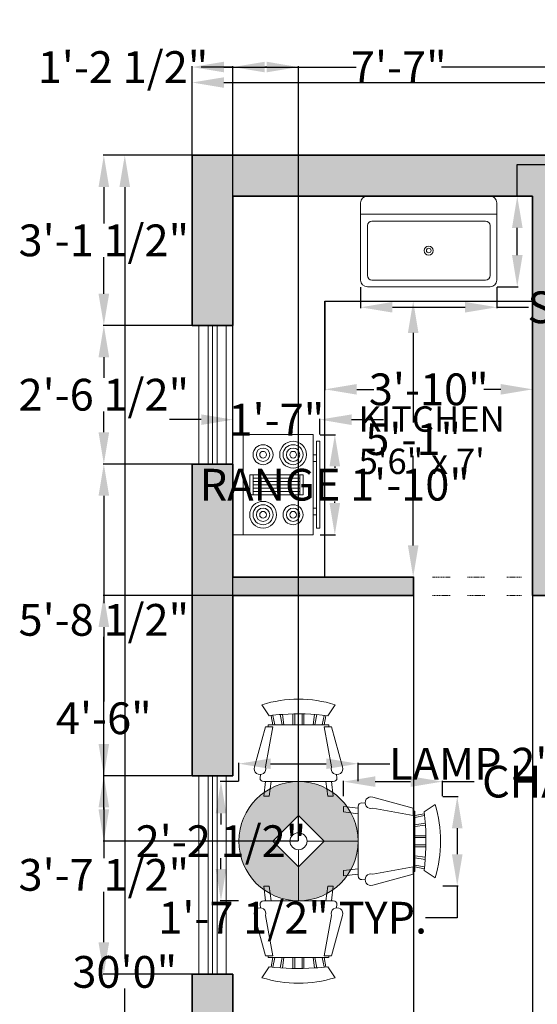
# Model space of a CAD drawing. Units: inches. Extents: x -8 to 329, y 10 to 430.
# Tile 3 of 4: x -8 to 106, y 213 to 430. Entities that reach past the tile are written whole.
import ezdxf

# ---------------------------------------------------------------- set-up
doc = ezdxf.new("R2010")
doc.units = ezdxf.units.IN
doc.header["$MEASUREMENT"] = 0
doc.linetypes.add('DASHED2', pattern=[0.375, 0.25, -0.125])
for name, color, linetype, lineweight in [('A-ANNO-DIMS', 2, 'Continuous', 18), ('A-AREA-IDEN', 7, 'Continuous', 18), ('A-EQPM', 8, 'Continuous', 18), ('A-FLOR-CASE', 9, 'Continuous', 25), ('A-FLOR-FIXT', 9, 'Continuous', 18), ('A-FURN', 8, 'Continuous', 18), ('A-GLAZ', 4, 'Continuous', 18), ('A-WALL', 7, 'Continuous', 35), ('A-WALL-OVHD', 8, 'DASHED2', 18), ('A-WALL-PATT', 253, 'Continuous', 13)]:
    doc.layers.add(name, color=color, linetype=linetype, lineweight=lineweight)
doc.layers.add('A-FURN-BASE-PATT', color=144, linetype='Continuous', lineweight=13, true_color=0x1e788f)
doc.styles.get("Standard").update_dxf_attribs({"font": 'arial.ttf'})
doc.dimstyles.get("Standard").update_dxf_attribs({"dimtxt": 7, "dimasz": 7, "dimexe": 0.18, "dimexo": 0.0625, "dimgap": 0.09, "dimtad": 0, "dimtih": 1, "dimtoh": 1, "dimdec": 0, "dimzin": 0, "dimdsep": 46, "dimlunit": 3, "dimtxsty": 'Standard', "dimcen": 0.09, "dimadec": 0, "dimazin": 0, "dimtfac": 1, "dimtdec": 0, "dimtofl": 0, "dimtmove": 0, "dimatfit": 3, "dimfxl": 1, "dimtolj": 1, "dimtzin": 0, "dimarcsym": 0})

# ---------------------------------------------------------------- blocks, each defined once
blk = doc.blocks.new('Lamp - Table')
for p, q in [((0, 7), (0, 1)), ((0, 3), (-3, 0)), ((3, 0), (0, 3)), ((-1, 0), (-7, 0)), ((-3, 0), (0, -3)), ((0, -3), (3, 0)), ((1, 0), (7, 0)), ((0, -1), (0, -7))]:
    blk.add_line(p, q)
for radius in [7, 1]:
    blk.add_circle((0, 0), radius)
blk = doc.blocks.new('Range-Oven - 30 in top')
for p, q in [((0, -3), (30, -3)), ((12, -6), (18, -6)), ((13, -20), (13, -6)), ((14, -6), (14, -20)), ((15, -20), (15, -6)), ((16, -6), (16, -20)), ((17, -20), (17, -6)), ((18, -20), (12, -20)), ((6, -24), (6, -25)), ((8, -25), (8, -24)), ((22, -25), (22, -24)), ((24, -24), (24, -25))]:
    blk.add_line(p, q)
for points in [[(0, -24), (0, 0), (30, 0), (30, -24)], [(12, -21), (12, -5), (18, -5), (18, -21)], [(2, -26), (2, -25), (28, -25), (28, -26)]]:
    blk.add_lwpolyline(points, close=True)
for centre, radius in [((6, -9), 4), ((6, -9), 3), ((6, -9), 2), ((6, -9), 1), ((24, -9), 3), ((24, -9), 2), ((24, -9), 1), ((24, -18), 4), ((6, -18), 3), ((6, -18), 2), ((6, -18), 1), ((24, -18), 3), ((24, -18), 2), ((24, -18), 1)]:
    blk.add_circle(centre, radius)
blk = doc.blocks.new('Sink-single - 30 in top')
blk.add_line((-15, -3.999996), (15, -3.999996))
for points in [[(-13.5, 0), (13.5, 0)], [(-15, -18.499996), (-15, -1.5)], [(15, -1.5), (15, -18.499996)], [(-13.5, -17.499996), (-13.5, -6.499996)], [(-12.5, -5.499996), (12.5, -5.499996)], [(13.5, -6.499996), (13.5, -17.499996)], [(12.5, -18.499996), (-12.5, -18.499996)], [(13.5, -19.999996), (-13.5, -19.999996)]]:
    blk.add_lwpolyline(points)
for radius in [1, 0.5]:
    blk.add_circle((0, -11.999996), radius)
for centre, radius, start, end in [((-13.5, -1.5), 1.5, 90, 180), ((13.5, -1.5), 1.5, 0, 90), ((-12.5, -6.499996), 1, 90, 180), ((12.5, -6.499996), 1, 0, 90), ((-13.5, -18.499996), 1.5, 180, 270), ((-12.5, -17.499996), 1, 180, 270), ((12.5, -17.499996), 1, 270, 0), ((13.5, -18.499996), 1.5, 270, 0)]:
    blk.add_arc(centre, radius, start, end)
blk = doc.blocks.new('Chair - Rocking')
for p, q in [((-8, -4.5), (-10, -1.5)), ((8, -4.5), (10, -1.5)), ((-7.5, -4.5), (-7, -7)), ((-6.5, -7), (-7.02225, -4.43)), ((-4.5, -7), (-4.96674, -4.19951)), ((-4, -7), (-4.40532, -4.16272)), ((-1.5, -4.05012), (-1.5, -7)), ((-1, -7), (-1, -4.05012)), ((1, -7), (1, -4.04655)), ((1.5, -4.05012), (1.5, -7)), ((4, -7), (4.40187, -4.18694)), ((4.5, -7), (4.96761, -4.19437)), ((6.5, -7), (7, -4.4057)), ((7.5, -4.5), (7, -7)), ((-9, -7.5), (-12, -18.49999)), ((-7, -7.5), (-9, -7.5)), ((-9, -18.49999), (-7, -7.5)), ((-8.23428, -6.99939), (-8.3093, -7.47958)), ((-8.23041, -7), (8.23915, -7)), ((7, -7.5), (9, -7.5)), ((9, -18.49999), (7, -7.5)), ((8.31071, -7.48854), (8.23449, -7.00073)), ((9, -7.5), (12, -18.49999)), ((-10.36644, -20.64523), (-10.5, -21.49999)), ((10.5, -21.49999), (10.3575, -20.58798)), ((-9, -22.49999), (-9.5, -26.49999)), ((0, -22.49999), (-9.5, -22.49999)), ((-8, -26.49999), (-7.5, -22.49999)), ((0, -22.49999), (9.5, -22.49999)), ((8, -26.49999), (7.5, -22.49999)), ((9, -22.49999), (9.5, -26.49999)), ((-9.5, -26.49999), (-8, -26.49999)), ((9.5, -26.49999), (8, -26.49999))]:
    blk.add_line(p, q)
for centre, radius, start, end in [((0, -34.08333), 34.08333, 72.93847, 107.0615), ((0, -68.25004), 64.25, 93.92211, 97.15267), ((0, -68.25004), 64.25, 82.84733, 93.92211), ((-10.5, -18.99999), 1.58114, 161.5651, 18.43495), ((10.5, -18.99999), 1.58114, 161.5651, 18.43495), ((-9.5, -21.49999), 1, 180, 270), ((9.5, -21.49999), 1, 270, 0)]:
    blk.add_arc(centre, radius, start, end)
blk = doc.blocks.new('*D15')
at = {"layer": 'A-ANNO-DIMS', "color": 0, "lineweight": -2, "transparency": 16777216}
for p, q in [((29.84, 399.76), (14.88, 399.76)), ((15.06, 392.76), (15.06, 223.43)), ((15.06, 46.76), (15.06, 216.1)), ((29.84, 39.76), (14.88, 39.76))]:
    blk.add_line(p, q, dxfattribs=at)
at = {"layer": 'A-ANNO-DIMS', "color": 0, "transparency": 16777216}
for points in [[(13.89, 392.76), (16.23, 392.76), (15.06, 399.76)], [(13.89, 46.76), (16.23, 46.76), (15.06, 39.76)]]:
    blk.add_solid(points, dxfattribs=at)
at = {"layer": 'Defpoints', "color": 0, "transparency": 16777216}
for p in [(29.9, 399.76), (15.06, 39.76), (29.9, 39.76)]:
    blk.add_point(p, dxfattribs=at)
at = {"layer": 'A-ANNO-DIMS', "color": 0, "transparency": 16777216, "insert": (15.06, 219.76), "char_height": 7, "attachment_point": 5}
blk.add_mtext('\\A1;30\'0"', dxfattribs=at)
blk = doc.blocks.new('*D16')
at = {"layer": 'A-ANNO-DIMS', "color": 0, "lineweight": -2, "transparency": 16777216}
for p, q in [((29.9, 399.83), (29.9, 415.98)), ((36.9, 415.8), (139.36, 415.8)), ((262.9, 415.8), (160.45, 415.8)), ((269.9, 399.83), (269.9, 415.98))]:
    blk.add_line(p, q, dxfattribs=at)
at = {"layer": 'A-ANNO-DIMS', "color": 0, "transparency": 16777216}
for points in [[(36.9, 416.96), (36.9, 414.63), (29.9, 415.8)], [(262.9, 416.96), (262.9, 414.63), (269.9, 415.8)]]:
    blk.add_solid(points, dxfattribs=at)
at = {"layer": 'Defpoints', "color": 0, "transparency": 16777216}
for p in [(269.9, 415.8), (29.9, 399.76), (269.9, 399.76)]:
    blk.add_point(p, dxfattribs=at)
at = {"layer": 'A-ANNO-DIMS', "color": 0, "transparency": 16777216, "insert": (149.9, 415.8), "char_height": 7, "attachment_point": 5}
blk.add_mtext('\\A1;20\'0"', dxfattribs=at)
blk = doc.blocks.new('*D22')
at = {"layer": 'A-ANNO-DIMS', "color": 0, "lineweight": -2, "transparency": 16777216}
for p, q in [((40.19, 261.77), (40.19, 265.83)), ((47.19, 265.65), (59.46, 265.65)), ((66.46, 261.77), (66.46, 265.83)), ((66.46, 265.65), (73.46, 265.65))]:
    blk.add_line(p, q, dxfattribs=at)
at = {"layer": 'A-ANNO-DIMS', "color": 0, "transparency": 16777216}
for points in [[(47.19, 266.81), (47.19, 264.48), (40.19, 265.65)], [(59.46, 266.81), (59.46, 264.48), (66.46, 265.65)]]:
    blk.add_solid(points, dxfattribs=at)
at = {"layer": 'Defpoints', "color": 0, "transparency": 16777216}
for p in [(66.46, 265.65), (40.19, 261.71), (66.46, 261.71)]:
    blk.add_point(p, dxfattribs=at)
at = {"layer": 'A-ANNO-DIMS', "color": 0, "transparency": 16777216, "insert": (105.53, 265.65), "char_height": 7, "attachment_point": 5}
blk.add_mtext('\\A1;LAMP 2\'-2 1/2"', dxfattribs=at)
blk = doc.blocks.new('*D23')
at = {"layer": 'A-ANNO-DIMS', "color": 0, "lineweight": -2, "transparency": 16777216}
for p, q in [((40.13, 261.71), (36.07, 261.71)), ((36.25, 254.71), (36.25, 252.28)), ((36.25, 242.44), (36.25, 244.86)), ((40.13, 235.44), (36.07, 235.44))]:
    blk.add_line(p, q, dxfattribs=at)
at = {"layer": 'A-ANNO-DIMS', "color": 0, "transparency": 16777216}
for points in [[(35.09, 254.71), (37.42, 254.71), (36.25, 261.71)], [(35.09, 242.44), (37.42, 242.44), (36.25, 235.44)]]:
    blk.add_solid(points, dxfattribs=at)
at = {"layer": 'Defpoints', "color": 0, "transparency": 16777216}
for p in [(36.25, 261.71), (40.19, 261.71), (40.19, 235.44)]:
    blk.add_point(p, dxfattribs=at)
at = {"layer": 'A-ANNO-DIMS', "color": 0, "transparency": 16777216, "insert": (36.25, 248.57), "char_height": 7, "attachment_point": 5}
blk.add_mtext('\\A1;2\'-2 1/2"', dxfattribs=at)
blk = doc.blocks.new('*D28')
at = {"layer": 'A-ANNO-DIMS', "color": 0, "lineweight": -2, "transparency": 16777216}
for p, q in [((63.23, 258.5), (63.23, 261.88)), ((70.23, 261.7), (78.03, 261.7)), ((85.03, 258.5), (85.03, 261.88)), ((85.03, 261.7), (92.03, 261.7))]:
    blk.add_line(p, q, dxfattribs=at)
at = {"layer": 'A-ANNO-DIMS', "color": 0, "transparency": 16777216}
for points in [[(70.23, 262.87), (70.23, 260.54), (63.23, 261.7)], [(78.03, 262.87), (78.03, 260.54), (85.03, 261.7)]]:
    blk.add_solid(points, dxfattribs=at)
at = {"layer": 'Defpoints', "color": 0, "transparency": 16777216}
for p in [(85.03, 261.7), (63.23, 258.43), (85.03, 258.43)]:
    blk.add_point(p, dxfattribs=at)
at = {"layer": 'A-ANNO-DIMS', "color": 0, "transparency": 16777216, "insert": (132.71, 261.7), "char_height": 7, "attachment_point": 5}
blk.add_mtext('\\A1;CHAIR 1\'-10" TYP.', dxfattribs=at)
blk = doc.blocks.new('*D29')
at = {"layer": 'A-ANNO-DIMS', "color": 0, "lineweight": -2, "transparency": 16777216}
for p, q in [((85.09, 258.43), (88.48, 258.43)), ((88.3, 251.43), (88.3, 245.71)), ((85.09, 238.71), (88.48, 238.71)), ((88.3, 238.71), (88.3, 231.71)), ((88.3, 231.71), (81.3, 231.71))]:
    blk.add_line(p, q, dxfattribs=at)
at = {"layer": 'A-ANNO-DIMS', "color": 0, "transparency": 16777216}
for points in [[(87.13, 251.43), (89.47, 251.43), (88.3, 258.43)], [(87.13, 245.71), (89.47, 245.71), (88.3, 238.71)]]:
    blk.add_solid(points, dxfattribs=at)
at = {"layer": 'Defpoints', "color": 0, "transparency": 16777216}
for p in [(85.03, 258.43), (85.03, 238.71), (88.3, 238.71)]:
    blk.add_point(p, dxfattribs=at)
at = {"layer": 'A-ANNO-DIMS', "color": 0, "transparency": 16777216, "insert": (52.05, 231.71), "char_height": 7, "attachment_point": 5}
blk.add_mtext('\\A1;1\'-7 1/2" TYP.', dxfattribs=at)
blk = doc.blocks.new('*D32')
at = {"layer": 'A-ANNO-DIMS', "color": 0, "lineweight": -2, "transparency": 16777216}
for p, q in [((126.75, 219.9), (117.76, 219.9)), ((117.94, 212.9), (117.94, 194.03)), ((117.94, 167.75), (117.94, 186.61)), ((126.75, 160.75), (117.76, 160.75))]:
    blk.add_line(p, q, dxfattribs=at)
at = {"layer": 'A-ANNO-DIMS', "color": 0, "transparency": 16777216}
for points in [[(116.77, 212.9), (119.1, 212.9), (117.94, 219.9)], [(116.77, 167.75), (119.1, 167.75), (117.94, 160.75)]]:
    blk.add_solid(points, dxfattribs=at)
at = {"layer": 'Defpoints', "color": 0, "transparency": 16777216}
for p in [(126.81, 219.9), (117.94, 160.75), (126.81, 160.75)]:
    blk.add_point(p, dxfattribs=at)
at = {"layer": 'A-ANNO-DIMS', "color": 0, "transparency": 16777216, "insert": (117.94, 190.32), "char_height": 7, "attachment_point": 5}
blk.add_mtext('\\A1;SOFA 4\'-11"', dxfattribs=at)
blk = doc.blocks.new('*D38')
at = {"layer": 'A-ANNO-DIMS', "color": 0, "lineweight": -2, "transparency": 16777216}
for p, q in [((58.08, 338.18), (61.51, 338.18)), ((61.33, 331.18), (61.33, 330.86)), ((61.33, 323.12), (61.33, 323.44)), ((58.08, 316.12), (61.51, 316.12))]:
    blk.add_line(p, q, dxfattribs=at)
at = {"layer": 'A-ANNO-DIMS', "color": 0, "transparency": 16777216}
for points in [[(60.16, 331.18), (62.5, 331.18), (61.33, 338.18)], [(60.16, 323.12), (62.5, 323.12), (61.33, 316.12)]]:
    blk.add_solid(points, dxfattribs=at)
at = {"layer": 'Defpoints', "color": 0, "transparency": 16777216}
for p in [(58.02, 338.18), (61.33, 338.18), (58.02, 316.12)]:
    blk.add_point(p, dxfattribs=at)
at = {"layer": 'A-ANNO-DIMS', "color": 0, "transparency": 16777216, "insert": (61.33, 327.15), "char_height": 7, "attachment_point": 5}
blk.add_mtext('\\A1;RANGE 1\'-10"', dxfattribs=at)
blk = doc.blocks.new('*D39')
at = {"layer": 'A-ANNO-DIMS', "color": 0, "lineweight": -2, "transparency": 16777216}
for p, q in [((31.9, 341.49), (24.9, 341.49)), ((38.9, 338.24), (38.9, 341.67)), ((58.02, 338.24), (58.02, 341.67)), ((65.02, 341.49), (72.02, 341.49))]:
    blk.add_line(p, q, dxfattribs=at)
at = {"layer": 'A-ANNO-DIMS', "color": 0, "transparency": 16777216}
for points in [[(31.9, 342.65), (31.9, 340.32), (38.9, 341.49)], [(65.02, 342.65), (65.02, 340.32), (58.02, 341.49)]]:
    blk.add_solid(points, dxfattribs=at)
at = {"layer": 'Defpoints', "color": 0, "transparency": 16777216}
for p in [(38.9, 341.49), (38.9, 338.18), (58.02, 338.18)]:
    blk.add_point(p, dxfattribs=at)
at = {"layer": 'A-ANNO-DIMS', "color": 0, "transparency": 16777216, "insert": (48.46, 341.49), "char_height": 7, "attachment_point": 5}
blk.add_mtext('\\A1;1\'-7"', dxfattribs=at)
blk = doc.blocks.new('*D40')
at = {"layer": 'A-ANNO-DIMS', "color": 0, "lineweight": -2, "transparency": 16777216}
for p, q in [((67.02, 370.7), (67.02, 366.08)), ((97.02, 370.7), (97.02, 366.08)), ((74.02, 366.26), (90.02, 366.26)), ((97.02, 366.26), (104.02, 366.26))]:
    blk.add_line(p, q, dxfattribs=at)
at = {"layer": 'A-ANNO-DIMS', "color": 0, "transparency": 16777216}
for points in [[(74.02, 367.43), (74.02, 365.1), (67.02, 366.26)], [(90.02, 367.43), (90.02, 365.1), (97.02, 366.26)]]:
    blk.add_solid(points, dxfattribs=at)
at = {"layer": 'Defpoints', "color": 0, "transparency": 16777216}
for p in [(67.02, 370.76), (97.02, 370.76), (97.02, 366.26)]:
    blk.add_point(p, dxfattribs=at)
at = {"layer": 'A-ANNO-DIMS', "color": 0, "transparency": 16777216, "insert": (126.17, 366.26), "char_height": 7, "attachment_point": 5}
blk.add_mtext('\\A1;SINK 2\'-6"', dxfattribs=at)
blk = doc.blocks.new('*D41')
at = {"layer": 'A-ANNO-DIMS', "color": 0, "lineweight": -2, "transparency": 16777216}
for p, q in [((101.52, 390.76), (101.52, 397.76)), ((101.52, 397.76), (108.52, 397.76)), ((97.09, 390.76), (101.7, 390.76)), ((101.52, 377.76), (101.52, 383.76)), ((97.09, 370.76), (101.7, 370.76))]:
    blk.add_line(p, q, dxfattribs=at)
at = {"layer": 'A-ANNO-DIMS', "color": 0, "transparency": 16777216}
for points in [[(100.36, 383.76), (102.69, 383.76), (101.52, 390.76)], [(100.36, 377.76), (102.69, 377.76), (101.52, 370.76)]]:
    blk.add_solid(points, dxfattribs=at)
at = {"layer": 'Defpoints', "color": 0, "transparency": 16777216}
for p in [(97.02, 390.76), (101.52, 390.76), (97.02, 370.76)]:
    blk.add_point(p, dxfattribs=at)
at = {"layer": 'A-ANNO-DIMS', "color": 0, "transparency": 16777216, "insert": (117.59, 397.76), "char_height": 7, "attachment_point": 5}
blk.add_mtext('\\A1;1\'-8"', dxfattribs=at)
blk = doc.blocks.new('*D50')
at = {"layer": 'A-ANNO-DIMS', "color": 0, "lineweight": -2, "transparency": 16777216}
for p, q in [((78.68, 302.7), (78.68, 20.13)), ((104.9, 302.7), (104.9, 20.13)), ((71.68, 20.31), (64.68, 20.31)), ((111.9, 20.31), (118.9, 20.31))]:
    blk.add_line(p, q, dxfattribs=at)
at = {"layer": 'A-ANNO-DIMS', "color": 0, "transparency": 16777216}
for points in [[(71.68, 21.48), (71.68, 19.15), (78.68, 20.31)], [(111.9, 21.48), (111.9, 19.15), (104.9, 20.31)]]:
    blk.add_solid(points, dxfattribs=at)
at = {"layer": 'Defpoints', "color": 0, "transparency": 16777216}
for p in [(78.68, 302.76), (104.9, 302.76), (104.9, 20.31)]:
    blk.add_point(p, dxfattribs=at)
at = {"layer": 'A-ANNO-DIMS', "color": 0, "transparency": 16777216, "insert": (91.79, 20.31), "char_height": 7, "attachment_point": 5}
blk.add_mtext('\\A1;2\'-2"', dxfattribs=at)
blk = doc.blocks.new('*D52')
at = {"layer": 'A-ANNO-DIMS', "color": 0, "lineweight": -2, "transparency": 16777216}
for p, q in [((29.84, 362.26), (10.27, 362.26)), ((10.45, 355.26), (10.45, 350.7)), ((10.45, 338.71), (10.45, 343.28)), ((29.84, 331.71), (10.27, 331.71))]:
    blk.add_line(p, q, dxfattribs=at)
at = {"layer": 'A-ANNO-DIMS', "color": 0, "transparency": 16777216}
for points in [[(9.28, 355.26), (11.62, 355.26), (10.45, 362.26)], [(9.28, 338.71), (11.62, 338.71), (10.45, 331.71)]]:
    blk.add_solid(points, dxfattribs=at)
at = {"layer": 'Defpoints', "color": 0, "transparency": 16777216}
for p in [(29.9, 362.26), (10.45, 331.71), (29.9, 331.71)]:
    blk.add_point(p, dxfattribs=at)
at = {"layer": 'A-ANNO-DIMS', "color": 0, "transparency": 16777216, "insert": (10.45, 346.99), "char_height": 7, "attachment_point": 5}
blk.add_mtext('\\A1;2\'-6 1/2"', dxfattribs=at)
blk = doc.blocks.new('*D53')
at = {"layer": 'A-ANNO-DIMS', "color": 0, "lineweight": -2, "transparency": 16777216}
for p, q in [((29.84, 263.01), (10.27, 263.01)), ((10.45, 256.01), (10.45, 244.86)), ((10.45, 226.28), (10.45, 237.44)), ((29.84, 219.28), (10.27, 219.28))]:
    blk.add_line(p, q, dxfattribs=at)
at = {"layer": 'A-ANNO-DIMS', "color": 0, "transparency": 16777216}
for points in [[(9.28, 256.01), (11.62, 256.01), (10.45, 263.01)], [(9.28, 226.28), (11.62, 226.28), (10.45, 219.28)]]:
    blk.add_solid(points, dxfattribs=at)
at = {"layer": 'Defpoints', "color": 0, "transparency": 16777216}
for p in [(29.9, 263.01), (10.45, 219.28), (29.9, 219.28)]:
    blk.add_point(p, dxfattribs=at)
at = {"layer": 'A-ANNO-DIMS', "color": 0, "transparency": 16777216, "insert": (10.45, 241.15), "char_height": 7, "attachment_point": 5}
blk.add_mtext('\\A1;3\'-7 1/2"', dxfattribs=at)
blk = doc.blocks.new('*D59')
at = {"layer": 'A-ANNO-DIMS', "color": 0, "lineweight": -2, "transparency": 16777216}
for p, q in [((29.84, 399.76), (10.27, 399.76)), ((10.45, 392.76), (10.45, 384.73)), ((10.45, 369.26), (10.45, 377.3)), ((29.84, 362.26), (10.27, 362.26))]:
    blk.add_line(p, q, dxfattribs=at)
at = {"layer": 'A-ANNO-DIMS', "color": 0, "transparency": 16777216}
for points in [[(9.28, 392.76), (11.62, 392.76), (10.45, 399.76)], [(9.28, 369.26), (11.62, 369.26), (10.45, 362.26)]]:
    blk.add_solid(points, dxfattribs=at)
at = {"layer": 'Defpoints', "color": 0, "transparency": 16777216}
for p in [(29.9, 399.76), (10.45, 362.26), (29.9, 362.26)]:
    blk.add_point(p, dxfattribs=at)
at = {"layer": 'A-ANNO-DIMS', "color": 0, "transparency": 16777216, "insert": (10.45, 381.01), "char_height": 7, "attachment_point": 5}
blk.add_mtext('\\A1;3\'-1 1/2"', dxfattribs=at)
blk = doc.blocks.new('*D60')
at = {"layer": 'A-ANNO-DIMS', "color": 0, "lineweight": -2, "transparency": 16777216}
for p, q in [((29.84, 331.71), (10.27, 331.71)), ((10.45, 324.71), (10.45, 301.07)), ((10.45, 270.01), (10.45, 293.65)), ((29.84, 263.01), (10.27, 263.01))]:
    blk.add_line(p, q, dxfattribs=at)
at = {"layer": 'A-ANNO-DIMS', "color": 0, "transparency": 16777216}
for points in [[(9.28, 324.71), (11.62, 324.71), (10.45, 331.71)], [(9.28, 270.01), (11.62, 270.01), (10.45, 263.01)]]:
    blk.add_solid(points, dxfattribs=at)
at = {"layer": 'Defpoints', "color": 0, "transparency": 16777216}
for p in [(29.9, 331.71), (10.45, 263.01), (29.9, 263.01)]:
    blk.add_point(p, dxfattribs=at)
at = {"layer": 'A-ANNO-DIMS', "color": 0, "transparency": 16777216, "insert": (10.45, 297.36), "char_height": 7, "attachment_point": 5}
blk.add_mtext('\\A1;5\'-8 1/2"', dxfattribs=at)
blk = doc.blocks.new('*D65')
at = {"layer": 'A-ANNO-DIMS', "color": 0, "lineweight": -2, "transparency": 16777216}
for p, q in [((29.9, 399.83), (29.9, 419.39)), ((36.9, 419.21), (66.07, 419.21)), ((113.96, 419.21), (84.8, 419.21)), ((120.96, 399.83), (120.96, 419.39))]:
    blk.add_line(p, q, dxfattribs=at)
at = {"layer": 'A-ANNO-DIMS', "color": 0, "transparency": 16777216}
for points in [[(36.9, 420.38), (36.9, 418.05), (29.9, 419.21)], [(113.96, 420.38), (113.96, 418.05), (120.96, 419.21)]]:
    blk.add_solid(points, dxfattribs=at)
at = {"layer": 'Defpoints', "color": 0, "transparency": 16777216}
for p in [(120.96, 419.21), (29.9, 399.76), (120.96, 399.76)]:
    blk.add_point(p, dxfattribs=at)
at = {"layer": 'A-ANNO-DIMS', "color": 0, "transparency": 16777216, "insert": (75.43, 419.21), "char_height": 7, "attachment_point": 5}
blk.add_mtext('\\A1;7\'-7"', dxfattribs=at)
blk = doc.blocks.new('*D70')
at = {"layer": 'A-ANNO-DIMS', "color": 0, "lineweight": -2, "transparency": 16777216}
for p, q in [((104.9, 306.7), (104.9, 20.13)), ((108.9, 306.7), (108.9, 20.13)), ((97.9, 20.31), (90.9, 20.31)), ((115.9, 20.31), (122.9, 20.31))]:
    blk.add_line(p, q, dxfattribs=at)
at = {"layer": 'A-ANNO-DIMS', "color": 0, "transparency": 16777216}
for points in [[(97.9, 21.48), (97.9, 19.15), (104.9, 20.31)], [(115.9, 21.48), (115.9, 19.15), (108.9, 20.31)]]:
    blk.add_solid(points, dxfattribs=at)
at = {"layer": 'Defpoints', "color": 0, "transparency": 16777216}
for p in [(104.9, 306.76), (108.9, 306.76), (108.9, 20.31)]:
    blk.add_point(p, dxfattribs=at)
at = {"layer": 'A-ANNO-DIMS', "color": 0, "transparency": 16777216, "insert": (132.29, 20.31), "char_height": 7, "attachment_point": 5}
blk.add_mtext('\\A1;0\'-4"', dxfattribs=at)
blk = doc.blocks.new('*D76')
at = {"layer": 'A-ANNO-DIMS', "color": 0, "lineweight": -2, "transparency": 16777216}
for p, q in [((38.9, 419.21), (31.9, 419.21)), ((38.9, 263.08), (38.9, 419.39)), ((46.33, 419.21), (45.9, 419.21)), ((53.33, 248.63), (53.33, 419.39))]:
    blk.add_line(p, q, dxfattribs=at)
at = {"layer": 'A-ANNO-DIMS', "color": 0, "transparency": 16777216}
for points in [[(45.9, 420.38), (45.9, 418.05), (38.9, 419.21)], [(46.33, 420.38), (46.33, 418.05), (53.33, 419.21)]]:
    blk.add_solid(points, dxfattribs=at)
at = {"layer": 'Defpoints', "color": 0, "transparency": 16777216}
for p in [(38.9, 419.21), (38.9, 263.01), (53.33, 248.57)]:
    blk.add_point(p, dxfattribs=at)
at = {"layer": 'A-ANNO-DIMS', "color": 0, "transparency": 16777216, "insert": (14.68, 419.21), "char_height": 7, "attachment_point": 5}
blk.add_mtext('\\A1;1\'-2 1/2"', dxfattribs=at)
blk = doc.blocks.new('*D77')
at = {"layer": 'A-ANNO-DIMS', "color": 0, "lineweight": -2, "transparency": 16777216}
for p, q in [((38.84, 302.76), (10.27, 302.76)), ((10.45, 295.76), (10.45, 279.33)), ((10.45, 255.57), (10.45, 272)), ((53.27, 248.57), (10.27, 248.57))]:
    blk.add_line(p, q, dxfattribs=at)
at = {"layer": 'A-ANNO-DIMS', "color": 0, "transparency": 16777216}
for points in [[(9.28, 295.76), (11.62, 295.76), (10.45, 302.76)], [(9.28, 255.57), (11.62, 255.57), (10.45, 248.57)]]:
    blk.add_solid(points, dxfattribs=at)
at = {"layer": 'Defpoints', "color": 0, "transparency": 16777216}
for p in [(10.45, 302.76), (38.9, 302.76), (53.33, 248.57)]:
    blk.add_point(p, dxfattribs=at)
at = {"layer": 'A-ANNO-DIMS', "color": 0, "transparency": 16777216, "insert": (10.45, 275.67), "char_height": 7, "attachment_point": 5}
blk.add_mtext('\\A1;4\'-6"', dxfattribs=at)
blk = doc.blocks.new('*D78')
at = {"layer": 'A-ANNO-DIMS', "color": 0, "lineweight": -2, "transparency": 16777216}
for p, q in [((59.15, 367.56), (59.15, 347.99)), ((104.9, 367.56), (104.9, 347.99)), ((66.15, 348.17), (69.91, 348.17)), ((97.9, 348.17), (94.14, 348.17))]:
    blk.add_line(p, q, dxfattribs=at)
at = {"layer": 'A-ANNO-DIMS', "color": 0, "transparency": 16777216}
for points in [[(66.15, 349.34), (66.15, 347.01), (59.15, 348.17)], [(97.9, 349.34), (97.9, 347.01), (104.9, 348.17)]]:
    blk.add_solid(points, dxfattribs=at)
at = {"layer": 'Defpoints', "color": 0, "transparency": 16777216}
for p in [(59.15, 367.62), (104.9, 367.62), (59.15, 348.17)]:
    blk.add_point(p, dxfattribs=at)
at = {"layer": 'A-ANNO-DIMS', "color": 0, "transparency": 16777216, "insert": (82.02, 348.17), "char_height": 7, "attachment_point": 5}
blk.add_mtext('\\A1;3\'-10"', dxfattribs=at)
blk = doc.blocks.new('*D79')
at = {"layer": 'A-ANNO-DIMS', "color": 0, "lineweight": -2, "transparency": 16777216}
for p, q in [((59.21, 367.62), (78.78, 367.62)), ((78.6, 360.62), (78.6, 340.86)), ((78.6, 313.76), (78.6, 333.53)), ((59.21, 306.76), (78.78, 306.76))]:
    blk.add_line(p, q, dxfattribs=at)
at = {"layer": 'A-ANNO-DIMS', "color": 0, "transparency": 16777216}
for points in [[(77.43, 360.62), (79.76, 360.62), (78.6, 367.62)], [(77.43, 313.76), (79.76, 313.76), (78.6, 306.76)]]:
    blk.add_solid(points, dxfattribs=at)
at = {"layer": 'Defpoints', "color": 0, "transparency": 16777216}
for p in [(59.15, 367.62), (59.15, 306.76), (78.6, 306.76)]:
    blk.add_point(p, dxfattribs=at)
at = {"layer": 'A-ANNO-DIMS', "color": 0, "transparency": 16777216, "insert": (78.6, 337.19), "char_height": 7, "attachment_point": 5}
blk.add_mtext('\\A1;5\'-1"', dxfattribs=at)

msp = doc.modelspace()

# ---------------------------------------------------------------- hatches: boundary and pattern name
at = {"layer": 'A-FURN-BASE-PATT'}
h = msp.add_hatch(color=256, dxfattribs=at)
h.dxf.hatch_style = 1
h.paths.add_polyline_path([(40.19, 248.57), (47.7, 248.57), (53.33, 254.2), (53.33, 261.71, 0.414214)])
h = msp.add_hatch(color=256, dxfattribs=at)
h.dxf.hatch_style = 1
h.paths.add_polyline_path([(53.33, 261.71), (53.33, 254.2), (58.96, 248.57), (66.46, 248.57, 0.414214)])
h = msp.add_hatch(color=256, dxfattribs=at)
h.dxf.hatch_style = 1
h.paths.add_polyline_path([(47.7, 248.57), (40.19, 248.57, 0.414214), (53.33, 235.44), (53.33, 242.94)])
h = msp.add_hatch(color=256, dxfattribs=at)
h.dxf.hatch_style = 1
h.paths.add_polyline_path([(53.33, 242.94), (53.33, 235.44, 0.414214), (66.46, 248.57), (58.96, 248.57)])
at = {"layer": 'A-WALL-PATT'}
h = msp.add_hatch(color=256, dxfattribs=at)
h.dxf.hatch_style = 1
h.paths.add_polyline_path([(29.9, 362.26), (38.9, 362.26), (38.9, 390.76), (104.9, 390.76), (104.9, 306.76), (104.9, 302.76), (108.9, 302.76), (108.9, 326.76), (150.9, 326.76), (150.9, 306.76), (154.9, 306.76), (154.9, 330.76), (151.5, 330.76), (133.34, 330.76), (108.9, 330.76), (108.9, 390.76), (120.96, 390.76), (120.96, 399.76), (29.9, 399.76)])
h = msp.add_hatch(color=256, dxfattribs=at)
h.dxf.hatch_style = 1
h.paths.add_polyline_path([(29.9, 263.01), (38.9, 263.01), (38.9, 302.76), (75.73, 302.76), (78.68, 302.76), (78.68, 306.76), (75.73, 306.76), (38.9, 306.76), (38.9, 331.71), (29.9, 331.71)])
h = msp.add_hatch(color=256, dxfattribs=at)
h.dxf.hatch_style = 1
h.paths.add_polyline_path([(38.9, 158.57), (38.47, 158.57), (38.47, 168.82), (37.62, 169.67), (37.62, 176.5), (38.47, 177.36), (38.47, 209.81), (38.9, 209.81), (38.9, 219.28), (29.9, 219.28), (29.9, 89.59), (38.9, 89.59), (38.9, 108.76), (47.18, 108.76), (47.18, 110.76), (47.18, 112.76), (38.9, 112.76)])

# ---------------------------------------------------------------- linework, layer by layer
at = {"layer": 'A-FLOR-CASE'}
for p, q in [((59.15, 367.62), (104.9, 367.62)), ((59.15, 306.76), (59.15, 367.62))]:
    msp.add_line(p, q, dxfattribs=at)
at = {"layer": 'A-GLAZ'}
for p, q in [((31.4, 362.26), (31.4, 331.71)), ((33.4, 362.26), (33.4, 331.71)), ((34.4, 362.26), (34.4, 331.71)), ((35.4, 362.26), (35.4, 331.71)), ((37.4, 362.26), (37.4, 331.71)), ((31.4, 263.01), (31.4, 219.28)), ((33.4, 263.01), (33.4, 219.28)), ((34.4, 263.01), (34.4, 219.28)), ((35.4, 263.01), (35.4, 219.28)), ((37.4, 263.01), (37.4, 219.28))]:
    msp.add_line(p, q, dxfattribs=at)
at = {"layer": 'A-WALL'}
for p, q in [((29.9, 399.76), (120.96, 399.76)), ((29.9, 362.26), (29.9, 399.76)), ((38.9, 390.76), (104.9, 390.76)), ((38.9, 362.26), (38.9, 390.76)), ((104.9, 306.76), (104.9, 390.76)), ((38.9, 362.26), (29.9, 362.26)), ((38.9, 331.71), (29.9, 331.71)), ((29.9, 263.01), (29.9, 331.71)), ((38.9, 306.76), (38.9, 331.71)), ((38.9, 306.76), (75.73, 306.76)), ((75.73, 306.76), (78.68, 306.76)), ((75.73, 306.76), (78.68, 306.76)), ((78.68, 302.76), (78.68, 306.76)), ((104.9, 306.76), (104.9, 302.76)), ((38.9, 302.76), (75.73, 302.76)), ((38.9, 263.01), (38.9, 302.76)), ((78.68, 302.76), (75.73, 302.76)), ((78.68, 302.76), (75.73, 302.76)), ((104.9, 302.76), (108.9, 302.76)), ((38.9, 263.01), (29.9, 263.01)), ((38.9, 219.28), (29.9, 219.28)), ((29.9, 89.59), (29.9, 219.28)), ((38.9, 112.76), (38.9, 219.28))]:
    msp.add_line(p, q, dxfattribs=at)
at = {"layer": 'A-WALL-OVHD'}
for p, q in [((82.87, 306.76), (86.74, 306.76)), ((82.87, 306.76), (86.74, 306.76)), ((90.54, 306.76), (94.38, 306.76)), ((90.54, 306.76), (94.38, 306.76)), ((90.54, 306.76), (94.38, 306.76)), ((99.22, 306.76), (102.47, 306.76)), ((99.22, 306.76), (102.47, 306.76)), ((99.22, 306.76), (102.47, 306.76)), ((86.74, 302.76), (82.87, 302.76)), ((86.74, 302.76), (82.87, 302.76)), ((94.38, 302.76), (90.54, 302.76)), ((94.38, 302.76), (90.54, 302.76)), ((102.47, 302.76), (99.22, 302.76)), ((102.47, 302.76), (99.22, 302.76))]:
    msp.add_line(p, q, dxfattribs=at)

# ---------------------------------------------------------------- block references
at = {"layer": 'A-EQPM', "xscale": 0.7353910637477178, "yscale": 0.7353910637477178, "zscale": 0.7353910637477178, "rotation": 90}
msp.add_blockref('Range-Oven - 30 in top', (38.9, 316.12), dxfattribs=at)
at = {"layer": 'A-FLOR-FIXT'}
msp.add_blockref('Sink-single - 30 in top', (82.02, 390.76), dxfattribs=at)
at = {"layer": 'A-FURN'}
for name, p, xscale, yscale, zscale in [('Chair - Rocking', (53.33, 279.87), 0.8073341388996443, 0.8073341388996443, 0.8073341388996443), ('Lamp - Table', (53.33, 248.57), 1.876408037315887, 1.876408037315887, 1.876408037315887)]:
    msp.add_blockref(name, p, dxfattribs=dict(at, xscale=xscale, yscale=yscale, zscale=zscale))
at = {"layer": 'A-FURN', "xscale": 0.8073341388996443, "yscale": 0.8073341388996443, "zscale": 0.8073341388996443}
for p, rotation in [((84.63, 248.57), 270), ((53.33, 217.27), 180)]:
    msp.add_blockref('Chair - Rocking', p, dxfattribs=dict(at, rotation=rotation))

# ---------------------------------------------------------------- texts
at = {"layer": 'A-AREA-IDEN', "insert": (66.57, 344.42), "char_height": 5.595, "attachment_point": 1}
msp.add_mtext_dynamic_manual_height_columns('KITCHEN\\P5\'6" x 7\'', width=164.8422, gutter_width=27.98, heights=[0], dxfattribs=at)

# ---------------------------------------------------------------- dimensions: what is measured, and where the dimension line sits
at = {"layer": 'A-ANNO-DIMS'}
for base, p1, p2, picture, middle in [((38.9, 419.21), (53.33, 248.57), (38.9, 263.01), '*D76', (14.68, 419.21)), ((120.96, 419.21), (29.9, 399.76), (120.96, 399.76), '*D65', (75.43, 419.21)), ((108.9, 20.31), (104.9, 306.76), (108.9, 306.76), '*D70', (132.29, 20.31)), ((104.9, 20.31), (78.68, 302.76), (104.9, 302.76), '*D50', (91.79, 20.31))]:
    dim = msp.add_linear_dim(base=base, p1=p1, p2=p2, dimstyle='Standard', override={"dimdec": 1, "dimlfac": 1, "dimrnd": 0, "dimzin": 1, "dimdsep": 46, "dimlunit": 4, "dimfrac": 2}, dxfattribs=at)
    dim.commit()
    dim.dimension.update_dxf_attribs({"geometry": picture, "text_midpoint": middle})
for base, p1, p2, text, override, picture, middle in [((269.9, 415.8), (29.9, 399.76), (269.9, 399.76), '<>0"', {"dimclrd": 0, "dimclre": 0, "dimclrt": 0}, '*D16', (149.9, 415.8)), ((97.02, 366.26), (67.02, 370.76), (97.02, 370.76), 'SINK <>', {"dimdec": 1, "dimlfac": 1, "dimrnd": 0, "dimzin": 1, "dimdsep": 46, "dimlunit": 4, "dimfrac": 2}, '*D40', (126.17, 366.26)), ((66.46, 265.65), (40.19, 261.71), (66.46, 261.71), 'LAMP <>', {"dimdec": 1, "dimlfac": 1, "dimrnd": 0, "dimzin": 1, "dimdsep": 46, "dimlunit": 4, "dimfrac": 2}, '*D22', (105.53, 265.65)), ((85.03, 261.7), (63.23, 258.43), (85.03, 258.43), 'CHAIR <> TYP.', {"dimdec": 1, "dimlfac": 1, "dimrnd": 0, "dimzin": 1, "dimdsep": 46, "dimlunit": 4, "dimfrac": 2}, '*D28', (132.71, 261.7))]:
    dim = msp.add_linear_dim(base=base, p1=p1, p2=p2, text=text, dimstyle='Standard', override=override, dxfattribs=at)
    dim.commit()
    dim.dimension.update_dxf_attribs({"geometry": picture, "text_midpoint": middle})
for base, p1, p2, angle, picture, middle in [((101.52, 390.76), (97.02, 370.76), (97.02, 390.76), 90, '*D41', (117.59, 397.76)), ((10.45, 362.26), (29.9, 399.76), (29.9, 362.26), 90, '*D59', (10.45, 381.01)), ((59.1483, 348.1748), (104.9006, 367.6248), (59.1483, 367.6248), 180, '*D78', (82.0244, 348.1748)), ((78.6, 306.76), (59.15, 367.62), (59.15, 306.76), 270, '*D79', (78.6, 337.19)), ((10.4506, 331.71), (29.9006, 362.2647), (29.9006, 331.71), 90, '*D52', (10.4506, 346.9873)), ((38.9, 341.49), (58.02, 338.18), (38.9, 338.18), 180, '*D39', (48.46, 341.49)), ((10.45, 263.01), (29.9, 331.71), (29.9, 263.01), 90, '*D60', (10.45, 297.36)), ((10.45, 302.76), (53.33, 248.57), (38.9, 302.76), 90, '*D77', (10.45, 275.67)), ((10.45, 219.28), (29.9, 263.01), (29.9, 219.28), 90, '*D53', (10.45, 241.15)), ((36.25, 261.71), (40.19, 235.44), (40.19, 261.71), 90, '*D23', (36.25, 248.57))]:
    dim = msp.add_linear_dim(base=base, p1=p1, p2=p2, angle=angle, dimstyle='Standard', override={"dimdec": 1, "dimlfac": 1, "dimrnd": 0, "dimzin": 1, "dimdsep": 46, "dimlunit": 4, "dimfrac": 2}, dxfattribs=at)
    dim.commit()
    dim.dimension.update_dxf_attribs({"geometry": picture, "text_midpoint": middle})
for base, p1, p2, angle, text, override, picture, middle in [((15.06, 39.76), (29.9, 399.76), (29.9, 39.76), 90, '<>0"', {"dimclrd": 0, "dimclre": 0, "dimclrt": 0}, '*D15', (15.06, 219.76)), ((61.33, 338.18), (58.02, 316.12), (58.02, 338.18), 90, 'RANGE <>', {"dimdec": 1, "dimlfac": 1, "dimrnd": 0, "dimzin": 1, "dimdsep": 46, "dimlunit": 4, "dimfrac": 2}, '*D38', (61.33, 327.15)), ((88.3, 238.71), (85.03, 258.43), (85.03, 238.71), 270, '<> TYP.', {"dimdec": 1, "dimlfac": 1, "dimrnd": 0, "dimzin": 1, "dimdsep": 46, "dimlunit": 4, "dimfrac": 2}, '*D29', (52.05, 231.71)), ((117.9359, 160.747), (126.8086, 219.8983), (126.8086, 160.747), 270, 'SOFA <>', {"dimdec": 1, "dimlfac": 1, "dimrnd": 0, "dimzin": 1, "dimdsep": 46, "dimlunit": 4, "dimfrac": 2}, '*D32', (117.9359, 190.3227))]:
    dim = msp.add_linear_dim(base=base, p1=p1, p2=p2, angle=angle, text=text, dimstyle='Standard', override=override, dxfattribs=at)
    dim.commit()
    dim.dimension.update_dxf_attribs({"geometry": picture, "text_midpoint": middle})

doc.saveas('drawing.dxf')
